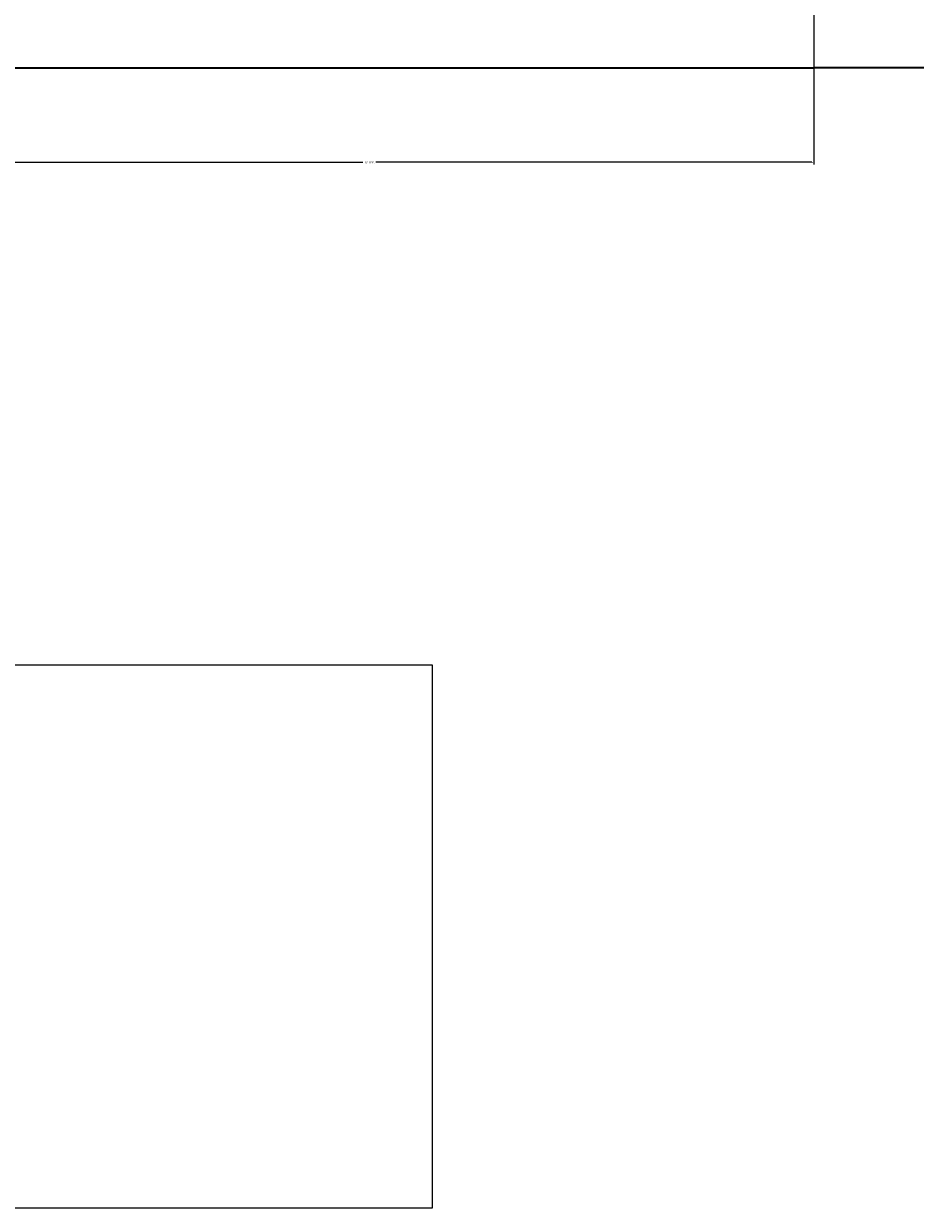
# Model space of a CAD drawing. Units: feet. Extents: x 1654 to 2985, y 1348 to 2230.
# Tile 4 of 53: x 1884 to 1956, y 1650 to 1746. Entities that reach past the tile are written whole.
import ezdxf

# ---------------------------------------------------------------- set-up
doc = ezdxf.new("R2010")
doc.units = ezdxf.units.FT
for name, color, linetype, lineweight in [('A-ANNO-DIMS', 2, 'Continuous', 18), ('A-FURN', 8, 'Continuous', 13), ('A-WALL', 7, 'Continuous', 35)]:
    doc.layers.add(name, color=color, linetype=linetype, lineweight=lineweight)
doc.styles.get("Standard").update_dxf_attribs({"font": 'arial.ttf'})
doc.dimstyles.get("Standard").update_dxf_attribs({"dimtxt": 0.18, "dimasz": 0.18, "dimexe": 0.18, "dimexo": 0.0625, "dimgap": 0.09, "dimtad": 0, "dimtih": 1, "dimtoh": 1, "dimdec": 4, "dimzin": 0, "dimdsep": 46, "dimtxsty": 'Standard', "dimcen": 0.09, "dimadec": 0, "dimazin": 0, "dimtfac": 1, "dimtdec": 4, "dimtofl": 0, "dimtmove": 0, "dimatfit": 3, "dimfxl": 1, "dimtolj": 1, "dimtzin": 0, "dimarcsym": 0})

# ---------------------------------------------------------------- blocks, each defined once
blk = doc.blocks.new('Bed - Queen')
for p, q in [((0, -80.00003), (0, 0)), ((0, 0), (59.99999, 0)), ((59.99999, 0), (59.99999, -80.00003)), ((7.99999, -1.2), (28.79998, -1.2)), ((7.99999, -14.4), (7.99999, -1.2)), ((28.79998, -1.2), (28.79998, -14.4)), ((31.19999, -1.2), (51.99999, -1.2)), ((31.19999, -14.4), (31.19999, -1.2)), ((51.99999, -1.2), (51.99999, -16.4)), ((0, -14.4), (44.8, -14.4)), ((59.99999, -29.6), (44.8, -14.4)), ((44.8, -14.4), (44.8, -29.6)), ((44.8, -16.8), (0, -16.8)), ((51.99999, -16.4), (46.79936, -16.4)), ((44.8, -29.6), (59.99999, -29.6)), ((59.99999, -80.00003), (0, -80.00003))]:
    blk.add_line(p, q)
blk = doc.blocks.new('*D75')
at = {"layer": 'A-ANNO-DIMS', "color": 0, "lineweight": -2, "transparency": 16777216}
for p, q in [((1876.092, 1751.192), (1876.092, 1734.425)), ((1948.092, 1751.192), (1948.092, 1734.425)), ((1876.272, 1734.605), (1911.565, 1734.605)), ((1947.912, 1734.605), (1912.62, 1734.605))]:
    blk.add_line(p, q, dxfattribs=at)
at = {"layer": 'A-ANNO-DIMS', "color": 0, "transparency": 16777216}
for points in [[(1876.272, 1734.635), (1876.272, 1734.575), (1876.092, 1734.605)], [(1947.912, 1734.635), (1947.912, 1734.575), (1948.092, 1734.605)]]:
    blk.add_solid(points, dxfattribs=at)
at = {"layer": 'Defpoints', "color": 0, "transparency": 16777216}
for p in [(1876.092, 1751.255), (1948.092, 1751.255), (1948.092, 1734.605)]:
    blk.add_point(p, dxfattribs=at)
at = {"layer": 'A-ANNO-DIMS', "color": 0, "transparency": 16777216, "insert": (1912.092, 1734.605), "char_height": 0.18, "attachment_point": 5}
blk.add_mtext('\\A1;72 TYP.', dxfattribs=at)

msp = doc.modelspace()

# ---------------------------------------------------------------- linework, layer by layer
at = {"layer": 'A-WALL'}
for p in [(1852.0924, 1742.2549), (1973.0924, 1742.2549)]:
    msp.add_line(p, (1948.0924, 1742.2549), dxfattribs=at)

# ---------------------------------------------------------------- block references
at = {"layer": 'A-FURN', "xscale": 0.7339343441631778, "yscale": 0.7339343441631778, "zscale": 0.7339343441631778, "rotation": 90}
msp.add_blockref('Bed - Queen', (1858.4494, 1649.8757), dxfattribs=at)

# ---------------------------------------------------------------- dimensions: what is measured, and where the dimension line sits
at = {"layer": 'A-ANNO-DIMS'}
dim = msp.add_linear_dim(base=(1948.0924, 1734.6049), p1=(1876.0924, 1751.2549), p2=(1948.0924, 1751.2549), text='<> TYP.', dimstyle='Standard', override={"dimdec": 0, "dimlfac": 1, "dimrnd": 0, "dimzin": 0, "dimdsep": 46, "dimlunit": 2}, dxfattribs=at)
dim.commit()
dim.dimension.update_dxf_attribs({"geometry": '*D75', "text_midpoint": (1912.0924, 1734.6049)})

doc.saveas('drawing.dxf')
